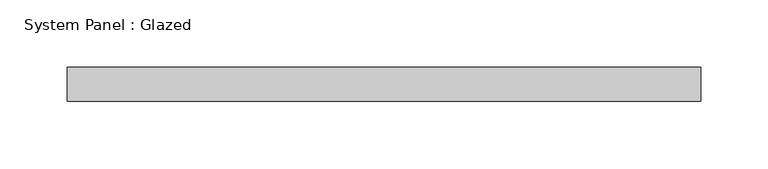
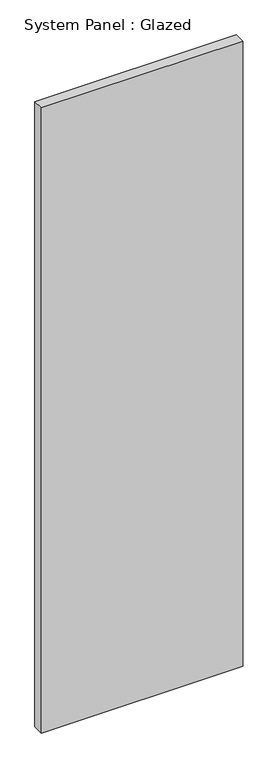
"""IFC4 building model written with IfcOpenShell, lengths in millimetres: plate geometry, System Panel : Glazed."""

from ifc_helpers import new_model, si_unit, origin, origin_with_axes, place, context, project, spatial, polyline, outline, extrude, source, transform, mapped, element, save


def system_panel_glazed_52f1247e(model_context):
    return source(origin(), model_context, "Body", "SweptSolid", [
        extrude(outline(polyline([(236.0083333, 19.05), (-236.0083333, 19.05), (-236.0083333, 44.45), (236.0083333, 44.45), (236.0083333, 19.05)])), origin_with_axes(), (0.0, 0.0, 1.0), 1548.2875727),
    ])


if __name__ == "__main__":
    model = new_model("IFC4")
    model_context = context("Model", 3, world=origin())
    ifc_project = project(units=[si_unit("LENGTHUNIT", "METRE", prefix="MILLI")], contexts=[model_context])
    site = spatial("IfcSite", under=ifc_project)
    building = spatial("IfcBuilding", under=site)
    placement = place(None, origin())
    system_panel_glazed_shape = system_panel_glazed_52f1247e(model_context)
    element("IfcPlate", 1, ObjectType="System Panel : Glazed", at=placement, inside=building, context=model_context, shape_type="MappedRepresentation", body=[
        mapped(system_panel_glazed_shape, transform((0.0, 0.0, 0.0), x_axis=(1.0, 0.0, 0.0), y_axis=(0.0, 1.0, 0.0), z_axis=(0.0, 0.0, 1.0))),
    ])
    save(model, "model.ifc")

# Revit data of these elements
# Type "System Panel : Glazed"
#   Construction Type Id = "GSP4R"
#   Analytic Construction = "1/8 in Pilkington single glazing"
#   Visual Light Transmittance = 0.9
#   Solar Heat Gain Coefficient = 0.86
#   Heat Transfer Coefficient (U) = 1.18115 BTU/(h·ft²·°F)
#   Define Thermal Properties by = 1
# Element 1 (IfcPlate, "System Panel : Glazed")
#   Materials on its faces: "Glass"
# Materials
#   "Glass": class "Glass", colour RGB 0 128 192, transparency 0.75, Description = "Soda Lime Glass", Cost = 0
